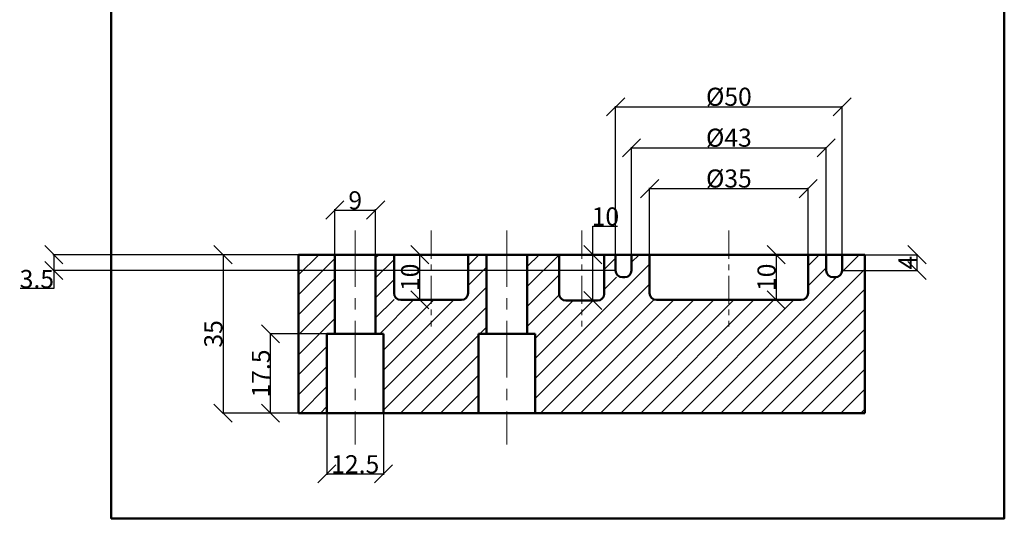
# Model space of a CAD drawing. Units: millimetres. Extents: x 145 to 386, y -112 to 157.
# Tile 1 of 2: x 145 to 363, y -112 to -2. Entities that reach past the tile are written whole.
import ezdxf

# ---------------------------------------------------------------- set-up
doc = ezdxf.new("R2010")
doc.units = ezdxf.units.MM
doc.header["$MEASUREMENT"] = 0
doc.linetypes.add('CENTER', pattern=[2, 1.25, -0.25, 0.25, -0.25])
for name, color, linetype, lineweight in [('M-CNTR', 1, 'CENTER', 18), ('M-DIMS', 2, 'Continuous', 25), ('M-HATC', 8, 'Continuous', 18), ('M-OUTL', 7, 'Continuous', 50), ('M-TTLB', 7, 'Continuous', 50)]:
    doc.layers.add(name, color=color, linetype=linetype, lineweight=lineweight)
doc.styles.get("Standard").update_dxf_attribs({"font": 'arial.ttf'})
doc.dimstyles.get("Standard").update_dxf_attribs({"dimtxt": 4, "dimasz": 4, "dimexe": 0.18, "dimexo": 0.0625, "dimgap": 0.09, "dimtad": 1, "dimtoh": 1, "dimdec": 0, "dimzin": 0, "dimdsep": 46, "dimtxsty": 'Standard', "dimblk": 'OBLIQUE', "dimcen": 0.09, "dimclre": 251, "dimadec": 0, "dimazin": 0, "dimtfac": 1, "dimtdec": 0, "dimtofl": 0, "dimtmove": 0, "dimatfit": 3, "dimfxl": 1, "dimtolj": 1, "dimtzin": 0, "dimarcsym": 0})

# ---------------------------------------------------------------- blocks, each defined once
blk = doc.blocks.new('_Oblique')
at = {"color": 0, "linetype": 'ByBlock', "lineweight": -2}
blk.add_line((-0.5, -0.5), (0.5, 0.5), dxfattribs=at)
blk = doc.blocks.new('*D2')
at = {"layer": 'Defpoints', "color": 0, "transparency": 16777216}
for p in [(207.01, -53.69), (190.32, -88.69), (207.01, -88.69)]:
    blk.add_point(p, dxfattribs=at)
at = {"layer": 'M-DIMS', "color": 0, "lineweight": -2, "transparency": 16777216}
for p, q in [((206.94, -53.69), (190.14, -53.69)), ((190.32, -53.69), (190.32, -88.69)), ((206.94, -88.69), (190.14, -88.69))]:
    blk.add_line(p, q, dxfattribs=at)
at = {"layer": 'M-DIMS', "color": 0, "lineweight": -2, "transparency": 16777216, "xscale": 4, "yscale": 4, "zscale": 4}
for p, rotation in [((190.32, -53.69), 90), ((190.32, -88.69), 270)]:
    blk.add_blockref('_Oblique', p, dxfattribs=dict(at, rotation=rotation))
at = {"layer": 'M-DIMS', "color": 0, "transparency": 16777216, "insert": (188.18, -71.19), "char_height": 4, "attachment_point": 5, "rotation": 90}
blk.add_mtext('\\A1;35', dxfattribs=at)
blk = doc.blocks.new('*D3')
at = {"layer": 'Defpoints', "color": 0, "transparency": 16777216}
for p in [(200.82, -71.19), (213.26, -71.19), (206.92, -88.69)]:
    blk.add_point(p, dxfattribs=at)
at = {"layer": 'M-DIMS', "color": 0, "lineweight": -2, "transparency": 16777216}
for p, q in [((213.19, -71.19), (200.64, -71.19)), ((200.82, -88.69), (200.82, -71.19)), ((206.86, -88.69), (200.64, -88.69))]:
    blk.add_line(p, q, dxfattribs=at)
at = {"layer": 'M-DIMS', "color": 0, "lineweight": -2, "transparency": 16777216, "xscale": 4, "yscale": 4, "zscale": 4}
for p, rotation in [((200.82, -71.19), 90), ((200.82, -88.69), 270)]:
    blk.add_blockref('_Oblique', p, dxfattribs=dict(at, rotation=rotation))
at = {"layer": 'M-DIMS', "color": 0, "transparency": 16777216, "insert": (198.69, -79.94), "char_height": 4, "attachment_point": 5, "rotation": 90}
blk.add_mtext('\\A1;17.5', dxfattribs=at)
blk = doc.blocks.new('*D4')
at = {"layer": 'Defpoints', "color": 0, "transparency": 16777216}
for p in [(224.01, -43.82), (215.02, -53.69), (224.01, -53.69)]:
    blk.add_point(p, dxfattribs=at)
at = {"layer": 'M-DIMS', "color": 0, "lineweight": -2, "transparency": 16777216}
for p, q in [((215.02, -53.63), (215.02, -43.64)), ((215.02, -43.82), (224.01, -43.82)), ((224.01, -53.63), (224.01, -43.64))]:
    blk.add_line(p, q, dxfattribs=at)
at = {"layer": 'M-DIMS', "color": 0, "lineweight": -2, "transparency": 16777216, "xscale": 4, "yscale": 4, "zscale": 4, "rotation": 180}
blk.add_blockref('_Oblique', (215.02, -43.82), dxfattribs=at)
at = {"layer": 'M-DIMS', "color": 0, "lineweight": -2, "transparency": 16777216, "xscale": 4, "yscale": 4, "zscale": 4}
blk.add_blockref('_Oblique', (224.01, -43.82), dxfattribs=at)
at = {"layer": 'M-DIMS', "color": 0, "transparency": 16777216, "insert": (219.51, -41.68), "char_height": 4, "attachment_point": 5}
blk.add_mtext('\\A1;9', dxfattribs=at)
blk = doc.blocks.new('*D5')
at = {"layer": 'Defpoints', "color": 0, "transparency": 16777216}
for p in [(213.26, -88.69), (225.76, -88.69), (225.76, -102.13)]:
    blk.add_point(p, dxfattribs=at)
at = {"layer": 'M-DIMS', "color": 0, "lineweight": -2, "transparency": 16777216}
for p, q in [((213.26, -88.75), (213.26, -102.31)), ((225.76, -88.75), (225.76, -102.31)), ((213.26, -102.13), (225.76, -102.13))]:
    blk.add_line(p, q, dxfattribs=at)
at = {"layer": 'M-DIMS', "color": 0, "lineweight": -2, "transparency": 16777216, "xscale": 4, "yscale": 4, "zscale": 4, "rotation": 180}
blk.add_blockref('_Oblique', (213.26, -102.13), dxfattribs=at)
at = {"layer": 'M-DIMS', "color": 0, "lineweight": -2, "transparency": 16777216, "xscale": 4, "yscale": 4, "zscale": 4}
blk.add_blockref('_Oblique', (225.76, -102.13), dxfattribs=at)
at = {"layer": 'M-DIMS', "color": 0, "transparency": 16777216, "insert": (219.51, -100), "char_height": 4, "attachment_point": 5}
blk.add_mtext('\\A1;12.5', dxfattribs=at)
blk = doc.blocks.new('*D6')
at = {"layer": 'Defpoints', "color": 0, "transparency": 16777216}
for p in [(233.77, -53.69), (233.77, -53.69), (233.77, -63.69)]:
    blk.add_point(p, dxfattribs=at)
at = {"layer": 'M-DIMS', "color": 0, "lineweight": -2, "transparency": 16777216}
for p, q in [((233.77, -63.69), (233.77, -53.69)), ((233.83, -53.69), (233.95, -53.69)), ((233.83, -63.69), (233.95, -63.69))]:
    blk.add_line(p, q, dxfattribs=at)
at = {"layer": 'M-DIMS', "color": 0, "lineweight": -2, "transparency": 16777216, "xscale": 4, "yscale": 4, "zscale": 4}
for p, rotation in [((233.77, -53.69), 90), ((233.77, -63.69), 270)]:
    blk.add_blockref('_Oblique', p, dxfattribs=dict(at, rotation=rotation))
at = {"layer": 'M-DIMS', "color": 0, "transparency": 16777216, "insert": (231.63, -58.69), "char_height": 4, "attachment_point": 5, "rotation": 90}
blk.add_mtext('\\A1;10', dxfattribs=at)
blk = doc.blocks.new('*D7')
at = {"layer": 'Defpoints', "color": 0, "transparency": 16777216}
for p in [(271.99, -53.69), (271.99, -53.69), (271.99, -63.83)]:
    blk.add_point(p, dxfattribs=at)
at = {"layer": 'M-DIMS', "color": 0, "lineweight": -2, "transparency": 16777216}
for p, q in [((271.99, -53.69), (271.99, -47.39)), ((271.99, -47.39), (277.42, -47.39)), ((271.92, -53.69), (271.81, -53.69)), ((271.99, -63.83), (271.99, -53.69)), ((271.92, -63.83), (271.81, -63.83))]:
    blk.add_line(p, q, dxfattribs=at)
at = {"layer": 'M-DIMS', "color": 0, "lineweight": -2, "transparency": 16777216, "xscale": 4, "yscale": 4, "zscale": 4}
for p, rotation in [((271.99, -53.69), 90), ((271.99, -63.83), 270)]:
    blk.add_blockref('_Oblique', p, dxfattribs=dict(at, rotation=rotation))
at = {"layer": 'M-DIMS', "color": 0, "transparency": 16777216, "insert": (274.75, -45.25), "char_height": 4, "attachment_point": 5}
blk.add_mtext('\\A1;10', dxfattribs=at)
blk = doc.blocks.new('*D8')
at = {"layer": 'Defpoints', "color": 0, "transparency": 16777216}
for p in [(332.01, -53.69), (327.01, -57.19), (343.55, -57.19)]:
    blk.add_point(p, dxfattribs=at)
at = {"layer": 'M-DIMS', "color": 0, "lineweight": -2, "transparency": 16777216}
for p, q in [((332.07, -53.69), (343.73, -53.69)), ((343.55, -53.69), (343.55, -57.19)), ((327.07, -57.19), (343.73, -57.19))]:
    blk.add_line(p, q, dxfattribs=at)
at = {"layer": 'M-DIMS', "color": 0, "lineweight": -2, "transparency": 16777216, "xscale": 4, "yscale": 4, "zscale": 4}
for p, rotation in [((343.55, -53.69), 90), ((343.55, -57.19), 270)]:
    blk.add_blockref('_Oblique', p, dxfattribs=dict(at, rotation=rotation))
at = {"layer": 'M-DIMS', "color": 0, "transparency": 16777216, "insert": (341.46, -55.44), "char_height": 4, "attachment_point": 5, "rotation": 90}
blk.add_mtext('\\A1;4', dxfattribs=at)
blk = doc.blocks.new('*D9')
at = {"layer": 'Defpoints', "color": 0, "transparency": 16777216}
for p in [(311.93, -53.69), (311.93, -63.69), (312.46, -63.69)]:
    blk.add_point(p, dxfattribs=at)
at = {"layer": 'M-DIMS', "color": 0, "lineweight": -2, "transparency": 16777216}
for p, q in [((311.99, -53.69), (312.64, -53.69)), ((312.46, -53.69), (312.46, -63.69)), ((311.99, -63.69), (312.64, -63.69))]:
    blk.add_line(p, q, dxfattribs=at)
at = {"layer": 'M-DIMS', "color": 0, "lineweight": -2, "transparency": 16777216, "xscale": 4, "yscale": 4, "zscale": 4}
for p, rotation in [((312.46, -53.69), 90), ((312.46, -63.69), 270)]:
    blk.add_blockref('_Oblique', p, dxfattribs=dict(at, rotation=rotation))
at = {"layer": 'M-DIMS', "color": 0, "transparency": 16777216, "insert": (310.33, -58.69), "char_height": 4, "attachment_point": 5, "rotation": 90}
blk.add_mtext('\\A1;10', dxfattribs=at)
blk = doc.blocks.new('*D10')
at = {"layer": 'Defpoints', "color": 0, "transparency": 16777216}
for p in [(319.51, -39.1), (284.51, -53.69), (319.51, -53.69)]:
    blk.add_point(p, dxfattribs=at)
at = {"layer": 'M-DIMS', "color": 0, "lineweight": -2, "transparency": 16777216}
for p, q in [((284.51, -53.63), (284.51, -38.92)), ((284.51, -39.1), (319.51, -39.1)), ((319.51, -53.63), (319.51, -38.92))]:
    blk.add_line(p, q, dxfattribs=at)
at = {"layer": 'M-DIMS', "color": 0, "lineweight": -2, "transparency": 16777216, "xscale": 4, "yscale": 4, "zscale": 4, "rotation": 180}
blk.add_blockref('_Oblique', (284.51, -39.1), dxfattribs=at)
at = {"layer": 'M-DIMS', "color": 0, "lineweight": -2, "transparency": 16777216, "xscale": 4, "yscale": 4, "zscale": 4}
blk.add_blockref('_Oblique', (319.51, -39.1), dxfattribs=at)
at = {"layer": 'M-DIMS', "color": 0, "transparency": 16777216, "insert": (302.01, -36.86), "char_height": 4, "attachment_point": 5}
blk.add_mtext('\\A1;%%C35', dxfattribs=at)
blk = doc.blocks.new('*D11')
at = {"layer": 'Defpoints', "color": 0, "transparency": 16777216}
for p in [(323.51, -30.08), (280.51, -53.69), (323.51, -53.69)]:
    blk.add_point(p, dxfattribs=at)
at = {"layer": 'M-DIMS', "color": 0, "lineweight": -2, "transparency": 16777216}
for p, q in [((280.51, -53.63), (280.51, -29.9)), ((280.51, -30.08), (323.51, -30.08)), ((323.51, -53.63), (323.51, -29.9))]:
    blk.add_line(p, q, dxfattribs=at)
at = {"layer": 'M-DIMS', "color": 0, "lineweight": -2, "transparency": 16777216, "xscale": 4, "yscale": 4, "zscale": 4, "rotation": 180}
blk.add_blockref('_Oblique', (280.51, -30.08), dxfattribs=at)
at = {"layer": 'M-DIMS', "color": 0, "lineweight": -2, "transparency": 16777216, "xscale": 4, "yscale": 4, "zscale": 4}
blk.add_blockref('_Oblique', (323.51, -30.08), dxfattribs=at)
at = {"layer": 'M-DIMS', "color": 0, "transparency": 16777216, "insert": (302.01, -27.84), "char_height": 4, "attachment_point": 5}
blk.add_mtext('\\A1;%%C43', dxfattribs=at)
blk = doc.blocks.new('*D12')
at = {"layer": 'Defpoints', "color": 0, "transparency": 16777216}
for p in [(327.01, -21.04), (277.01, -53.69), (327.01, -53.69)]:
    blk.add_point(p, dxfattribs=at)
at = {"layer": 'M-DIMS', "color": 0, "lineweight": -2, "transparency": 16777216}
for p, q in [((277.01, -53.63), (277.01, -20.86)), ((277.01, -21.04), (327.01, -21.04)), ((327.01, -53.63), (327.01, -20.86))]:
    blk.add_line(p, q, dxfattribs=at)
at = {"layer": 'M-DIMS', "color": 0, "lineweight": -2, "transparency": 16777216, "xscale": 4, "yscale": 4, "zscale": 4, "rotation": 180}
blk.add_blockref('_Oblique', (277.01, -21.04), dxfattribs=at)
at = {"layer": 'M-DIMS', "color": 0, "lineweight": -2, "transparency": 16777216, "xscale": 4, "yscale": 4, "zscale": 4}
blk.add_blockref('_Oblique', (327.01, -21.04), dxfattribs=at)
at = {"layer": 'M-DIMS', "color": 0, "transparency": 16777216, "insert": (302.01, -18.8), "char_height": 4, "attachment_point": 5}
blk.add_mtext('\\A1;%%C50', dxfattribs=at)
blk = doc.blocks.new('*D33')
at = {"layer": 'Defpoints', "color": 0, "transparency": 16777216}
for p in [(277.01, -53.69), (152.95, -57.19), (277.01, -57.19)]:
    blk.add_point(p, dxfattribs=at)
at = {"layer": 'M-DIMS', "color": 251, "lineweight": -2, "transparency": 16777216}
for p, q in [((276.94, -53.69), (152.77, -53.69)), ((276.94, -57.19), (152.77, -57.19))]:
    blk.add_line(p, q, dxfattribs=at)
at = {"layer": 'M-DIMS', "color": 0, "lineweight": -2, "transparency": 16777216}
for p, q in [((152.95, -53.69), (152.95, -57.19)), ((152.95, -57.19), (152.95, -61.19)), ((152.95, -61.19), (145.55, -61.19))]:
    blk.add_line(p, q, dxfattribs=at)
at = {"layer": 'M-DIMS', "color": 0, "lineweight": -2, "transparency": 16777216, "xscale": 4, "yscale": 4, "zscale": 4}
for p, rotation in [((152.95, -53.69), 90), ((152.95, -57.19), 270)]:
    blk.add_blockref('_Oblique', p, dxfattribs=dict(at, rotation=rotation))
at = {"layer": 'M-DIMS', "color": 0, "transparency": 16777216, "insert": (149.21, -59.06), "char_height": 4, "attachment_point": 5}
blk.add_mtext('\\A1;3.5', dxfattribs=at)

msp = doc.modelspace()

# ---------------------------------------------------------------- hatches: boundary and pattern name
at = {"layer": 'M-HATC'}
h = msp.add_hatch(dxfattribs=at)
h.set_pattern_fill('ANSI31', color=256, scale=25)
h.paths.add_polyline_path([(215.02, -53.69), (207.01, -53.69), (207.01, -88.69), (213.26, -88.69), (213.26, -71.19), (215.02, -71.19)])
h.paths.add_polyline_path([(246.76, -71.19), (248.51, -71.19), (248.51, -53.69), (244.45, -53.69), (244.45, -63.69), (228.07, -63.69), (228.07, -53.69), (224.01, -53.69), (224.01, -71.19), (225.76, -71.19), (225.76, -88.69), (246.76, -88.69)])
h.paths.add_polyline_path([(332.01, -53.69), (327.01, -53.69), (327.01, -58.69), (323.51, -58.69), (323.51, -53.69), (319.51, -53.69), (319.51, -63.69), (284.51, -63.69), (284.51, -53.69), (280.51, -53.69), (280.51, -58.69), (277.01, -58.69), (277.01, -53.69), (274.51, -53.69), (274.51, -63.83), (264.51, -63.83), (264.51, -53.69), (257.51, -53.69), (257.51, -71.19), (259.26, -71.19), (259.26, -88.69), (332.01, -88.69)])

# ---------------------------------------------------------------- linework, layer by layer
at = {"layer": 'M-CNTR', "ltscale": 10}
for p, q in [((219.51, -48.33), (219.51, -95.66)), ((253.01, -48.33), (253.01, -95.66))]:
    msp.add_line(p, q, dxfattribs=at)
at = {"layer": 'M-CNTR', "ltscale": 5}
for p, q in [((236.26, -48.33), (236.26, -69.53)), ((269.51, -48.33), (269.51, -69.53)), ((302.01, -48.33), (302.01, -69.53))]:
    msp.add_line(p, q, dxfattribs=at)
at = {"layer": 'M-OUTL'}
for p, q in [((207.01, -53.69), (207.01, -88.69)), ((207.01, -53.69), (332.01, -53.69)), ((215.02, -53.69), (215.02, -71.19)), ((224.01, -53.69), (224.01, -71.19)), ((228.07, -53.69), (228.07, -62.19)), ((244.45, -53.69), (244.45, -62.19)), ((248.51, -53.69), (248.51, -71.19)), ((257.51, -53.69), (257.51, -71.19)), ((264.51, -53.69), (264.51, -62.33)), ((274.51, -53.69), (274.51, -62.33)), ((277.01, -57.19), (277.01, -53.69)), ((280.51, -57.19), (280.51, -53.69)), ((284.51, -53.69), (284.51, -62.19)), ((319.51, -53.69), (319.51, -62.19)), ((323.51, -53.69), (323.51, -57.19)), ((327.01, -53.69), (327.01, -57.19)), ((332.01, -88.69), (332.01, -53.69)), ((278.51, -58.69), (279.01, -58.69)), ((325.01, -58.69), (325.51, -58.69)), ((229.57, -63.69), (242.95, -63.69)), ((266.01, -63.83), (273.01, -63.83)), ((286.01, -63.69), (318.01, -63.69)), ((213.26, -71.19), (213.26, -88.69)), ((213.26, -71.19), (225.76, -71.19)), ((225.76, -71.19), (225.76, -88.69)), ((246.76, -71.19), (246.76, -88.69)), ((246.76, -71.19), (259.26, -71.19)), ((259.26, -71.19), (259.26, -88.69)), ((207.01, -88.69), (332.01, -88.69))]:
    msp.add_line(p, q, dxfattribs=at)
for centre, start, end in [((278.51, -57.19), 180, 270), ((279.01, -57.19), 270, 0), ((325.01, -57.19), 180, 270), ((325.51, -57.19), 270, 0), ((229.57, -62.19), 180, 270), ((242.95, -62.19), 270, 0), ((266.01, -62.33), 180, 270), ((273.01, -62.33), 270, 0), ((286.01, -62.19), 180, 270), ((318.01, -62.19), 270, 0)]:
    msp.add_arc(centre, 1.5, start, end, dxfattribs=at)
at = {"layer": 'M-TTLB'}
msp.add_lwpolyline([(165.63, 139.25), (362.83, 139.25), (362.83, -111.95), (165.63, -111.95)], close=True, dxfattribs=at)

# ---------------------------------------------------------------- dimensions: what is measured, and where the dimension line sits
at = {"layer": 'M-DIMS'}
for base, p1, p2, picture, middle in [((327.01, -21.04), (277.01, -53.69), (327.01, -53.69), '*D12', (302.01, -18.8)), ((323.51, -30.08), (280.51, -53.69), (323.51, -53.69), '*D11', (302.01, -27.84)), ((319.51, -39.1), (284.51, -53.69), (319.51, -53.69), '*D10', (302.01, -36.86))]:
    dim = msp.add_linear_dim(base=base, p1=p1, p2=p2, text='%%C<>', dimstyle='Standard', override={"dimclrd": 0, "dimclre": 0, "dimclrt": 0}, dxfattribs=at)
    dim.commit()
    dim.dimension.update_dxf_attribs({"geometry": picture, "text_midpoint": middle})
for base, p1, p2, override, picture, middle in [((224.01, -43.82), (215.02, -53.69), (224.01, -53.69), {"dimclrd": 0, "dimclre": 0, "dimclrt": 0}, '*D4', (219.51, -41.68)), ((225.76, -102.13), (213.26, -88.69), (225.76, -88.69), {"dimdec": 1, "dimclrd": 0, "dimclre": 0, "dimclrt": 0}, '*D5', (219.51, -100))]:
    dim = msp.add_linear_dim(base=base, p1=p1, p2=p2, dimstyle='Standard', override=override, dxfattribs=at)
    dim.commit()
    dim.dimension.update_dxf_attribs({"geometry": picture, "text_midpoint": middle})
dim = msp.add_linear_dim(base=(271.99, -53.69), p1=(271.99, -63.83), p2=(271.99, -53.69), angle=90, dimstyle='Standard', override={"dimclrd": 0, "dimclre": 0, "dimclrt": 0}, dxfattribs=at)
dim.commit()
dim.dimension.update_dxf_attribs({"geometry": '*D7', "text_midpoint": (274.75, -47.39), "dimtype": 160})
for base, p1, p2, override, picture, middle in [((152.95, -57.19), (277.01, -53.69), (277.01, -57.19), {"dimdec": 1, "dimlfac": 1, "dimrnd": 0, "dimzin": 0, "dimdsep": 46, "dimlunit": 2}, '*D33', (149.21, -59.06)), ((190.32, -88.69), (207.01, -53.69), (207.01, -88.69), {"dimclrd": 0, "dimclre": 0, "dimclrt": 0}, '*D2', (188.18, -71.19)), ((233.77, -53.69), (233.77, -63.69), (233.77, -53.69), {"dimclrd": 0, "dimclre": 0, "dimclrt": 0}, '*D6', (231.63, -58.69)), ((312.46, -63.69), (311.93, -53.69), (311.93, -63.69), {"dimclrd": 0, "dimclre": 0, "dimclrt": 0}, '*D9', (310.33, -58.69)), ((343.5521245, -57.19221853), (332.00732943, -53.69221853), (327.00732943, -57.19221853), {"dimclrd": 0, "dimclre": 0, "dimclrt": 0}, '*D8', (341.4621245, -55.44221853)), ((200.82, -71.19), (206.92, -88.69), (213.26, -71.19), {"dimdec": 1, "dimclrd": 0, "dimclre": 0, "dimclrt": 0}, '*D3', (198.69, -79.94))]:
    dim = msp.add_linear_dim(base=base, p1=p1, p2=p2, angle=90, dimstyle='Standard', override=override, dxfattribs=at)
    dim.commit()
    dim.dimension.update_dxf_attribs({"geometry": picture, "text_midpoint": middle})

doc.saveas('drawing.dxf')
